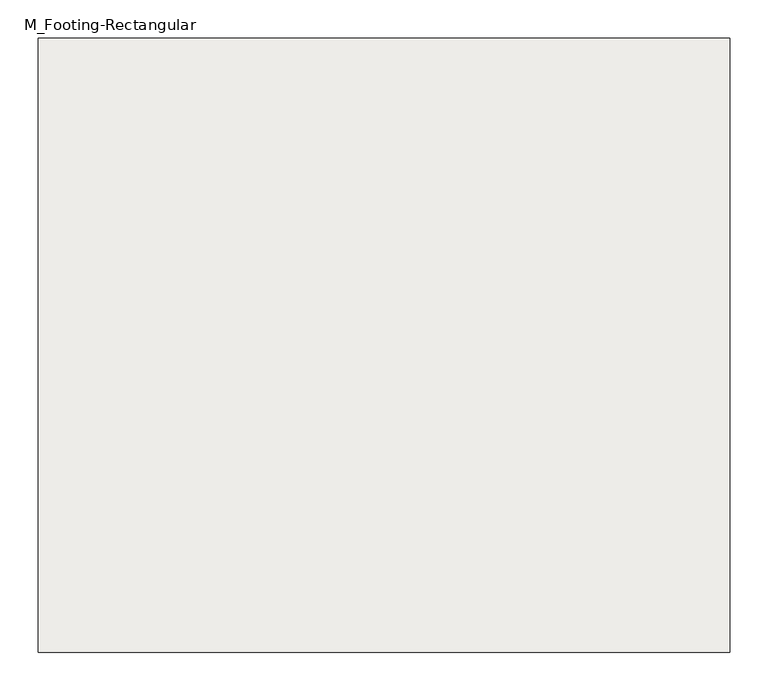
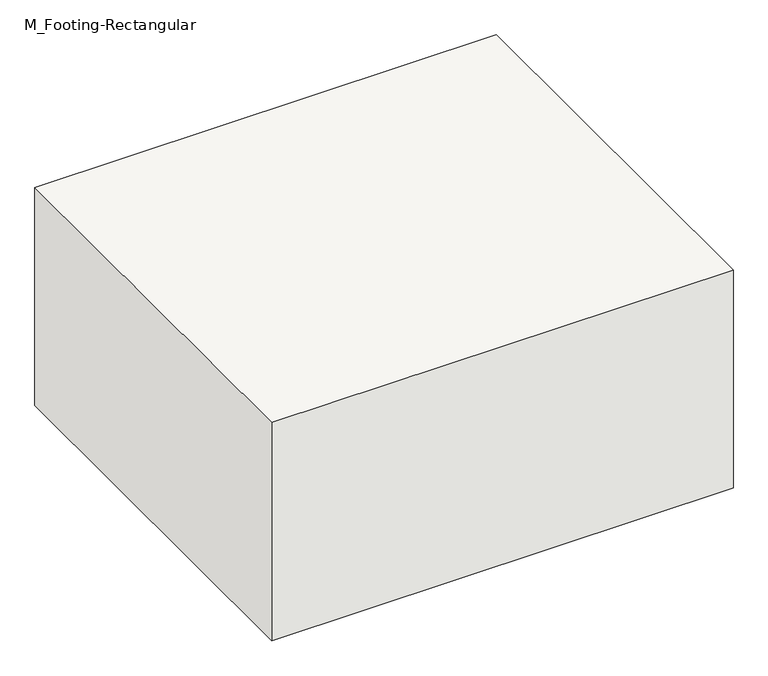
"""IFC4 building model written with IfcOpenShell, lengths in millimetres: slab geometry, M_Footing-Rectangular."""

from ifc_helpers import new_model, si_unit, frame, origin, place, context, project, spatial, polyline, outline, extrude, source, transform, mapped, element, save


def m_footing_rectangular_f0562f77(model_context):
    return source(origin(), model_context, "Body", "SweptSolid", [
        extrude(outline(polyline([(450.0, 400.0), (450.0, -400.0), (-450.0, -400.0), (-450.0, 400.0), (450.0, 400.0)])), frame((0.0, 0.0, -450.0), z_axis=(0.0, 0.0, 1.0), x_axis=(1.0, 0.0, 0.0)), (0.0, 0.0, 1.0), 450.0),
    ])


if __name__ == "__main__":
    model = new_model("IFC4")
    model_context = context("Model", 3, world=origin())
    ifc_project = project(units=[si_unit("LENGTHUNIT", "METRE", prefix="MILLI")], contexts=[model_context])
    site = spatial("IfcSite", under=ifc_project)
    building = spatial("IfcBuilding", under=site)
    placement = place(None, origin())
    m_footing_rectangular_shape = m_footing_rectangular_f0562f77(model_context)
    element("IfcSlab", 1, ObjectType="M_Footing-Rectangular", at=placement, inside=building, context=model_context, shape_type="MappedRepresentation", body=[
        mapped(m_footing_rectangular_shape, transform((0.0, 0.0, 0.0), x_axis=(1.0, 0.0, 0.0), y_axis=(0.0, 1.0, 0.0), z_axis=(0.0, 0.0, 1.0))),
    ])
    save(model, "model.ifc")

# Revit data of these elements
# Type "M_Footing-Rectangular"
#   Width = 2' - 11.43307"
#   Length = 2' - 7.49606"
#   Foundation Thickness = 1' - 5.71654"
#   Structural Material [instance default] = Concrete, Cast-in-Place gray
#   Assembly Code = ""
# Element 1 (IfcSlab, "M_Footing-Rectangular")
#   Materials on its faces: "Concrete, Cast-in-Place gray"
# Materials
#   "Concrete, Cast-in-Place gray": class "Concrete", colour RGB 192 192 192, transparency 0, Description = "Cast-in-place concrete", Cost = 0
